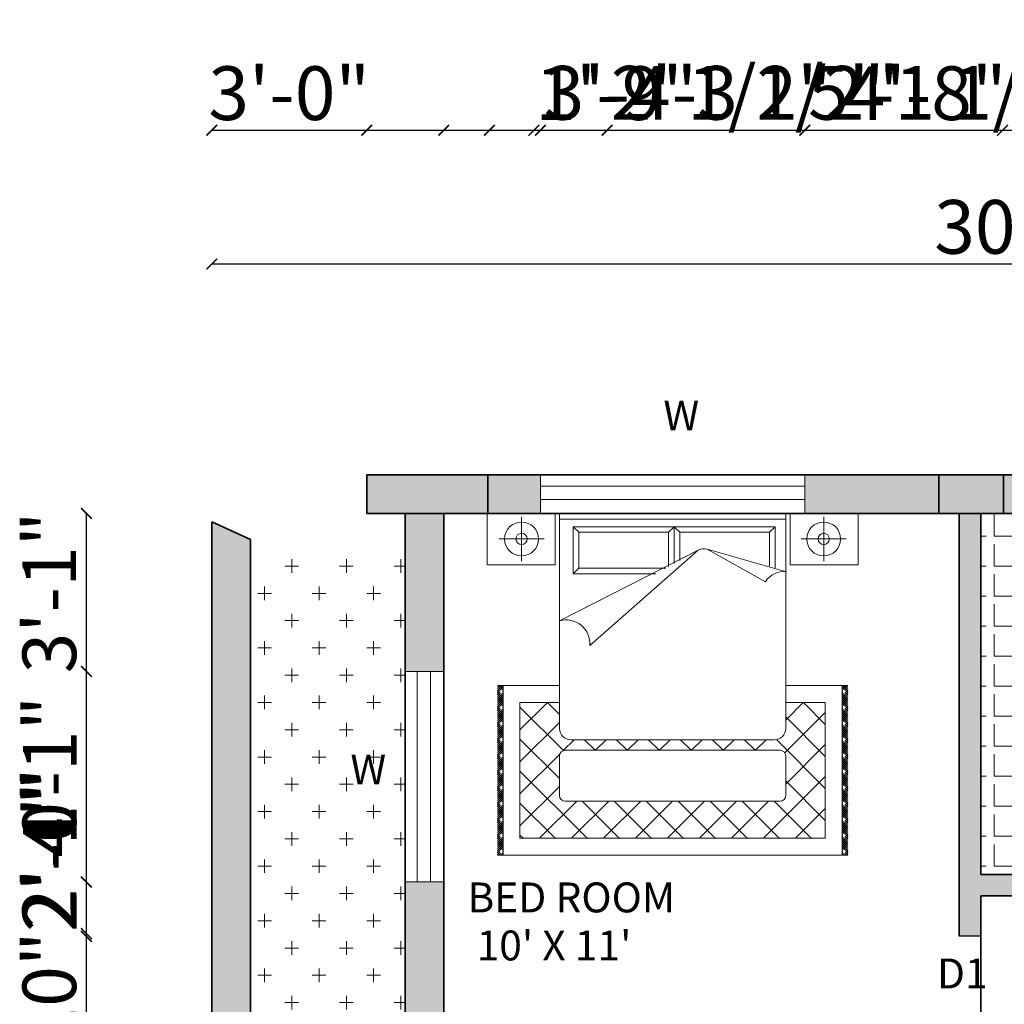
# Model space of a CAD drawing. Units: inches. Extents: x 1858 to 2399, y 1317 to 1943.
# Tile 3 of 8: x 1869 to 2098, y 1714 to 1943. Entities that reach past the tile are written whole.
import ezdxf

# ---------------------------------------------------------------- set-up
doc = ezdxf.new("R2010")
doc.units = ezdxf.units.IN
for name, color, linetype, lineweight in [('A-ANNO-DIMS', 2, 'Continuous', 18), ('A-ANNO-TEXT', 7, 'Continuous', 18), ('A-AREA-IDEN', 7, 'Continuous', 18), ('A-COLS', 7, 'Continuous', 35), ('A-COLS-PATT', 5, 'Continuous', 13), ('A-DOOR', 4, 'Continuous', 25), ('A-FLOR-PATT', 8, 'Continuous', 13), ('A-WALL', 7, 'Continuous', 35), ('A-WALL-PATT', 1, 'Continuous', 13), ('beds', 15, 'Continuous', 18), ('L-SITE-PATT', 8, 'Continuous', 13), ('window', 4, 'Continuous', 18)]:
    doc.layers.add(name, color=color, linetype=linetype, lineweight=lineweight)
doc.styles.get("Standard").update_dxf_attribs({"font": 'arial.ttf'})
doc.dimstyles.new('ISO-25', dxfattribs={"dimtxt": 12.5, "dimasz": 2.5, "dimexe": 1.25, "dimexo": 0.625, "dimtad": 1, "dimdec": 0, "dimlunit": 4, "dimtxsty": 'Standard', "dimblk": 'ARCHTICK', "dimcen": 2.5, "dimse1": 1, "dimse2": 1, "dimclrd": 3, "dimclrt": 4, "dimadec": 0, "dimazin": 0, "dimtfac": 1, "dimtdec": 0, "dimtmove": 0, "dimatfit": 3, "dimfxl": 1, "dimarcsym": 0})

# ---------------------------------------------------------------- blocks, each defined once
blk = doc.blocks.new('A$C4CB008C5')
for p, q in [((0, 3.0188), (0.6, 3.0188)), ((0, 2.5688), (0, 3.0188)), ((0.3042, 2.5999), (0.3042, 2.9921)), ((0.6, 3.0188), (0.6, 2.5688)), ((0.6397, 1.1213), (0.6397, 3.0213)), ((0.6397, 3.0213), (2.6397, 3.0213)), ((0.6397, 2.9713), (2.6397, 2.9713)), ((2.6397, 3.0213), (2.6397, 1.1213)), ((3.2794, 3.0188), (2.6794, 3.0188)), ((2.6794, 3.0188), (2.6794, 2.5688)), ((2.9753, 2.5999), (2.9753, 2.9921)), ((3.2794, 2.5688), (3.2794, 3.0188)), ((0.7588, 2.9048), (2.5468, 2.9048)), ((0.7588, 2.4886), (0.7588, 2.9048)), ((0.7588, 2.9048), (0.8088, 2.8548)), ((1.6028, 2.8548), (1.6528, 2.9048)), ((1.6528, 2.9048), (1.6528, 2.5791)), ((1.6528, 2.9048), (1.7028, 2.8548)), ((2.4968, 2.8548), (2.5468, 2.9048)), ((2.5468, 2.9048), (2.5468, 2.5398)), ((0.1057, 2.796), (0.5033, 2.796)), ((0.8088, 2.8548), (1.6028, 2.8548)), ((0.8088, 2.5386), (0.8088, 2.8548)), ((1.6028, 2.8548), (1.6028, 2.5513)), ((1.7028, 2.8548), (1.7028, 2.6069)), ((1.7028, 2.8548), (2.4968, 2.8548)), ((2.4968, 2.8548), (2.4968, 2.5563)), ((3.1738, 2.796), (2.7761, 2.796)), ((1.946, 2.7052), (2.6461, 2.507)), ((1.946, 2.7052), (2.4598, 2.4178)), ((0.6397, 2.0713), (1.866, 2.6977)), ((0.9063, 1.8539), (1.866, 2.6977)), ((0.6, 2.5688), (0, 2.5688)), ((0.8088, 2.5386), (0.7588, 2.4886)), ((1.58, 2.5386), (0.8088, 2.5386)), ((2.6794, 2.5688), (3.2794, 2.5688)), ((1.4901, 2.4886), (0.7588, 2.4886)), ((0.9071, 1.8666), (0.9192, 1.8666)), ((0.0897, 1.5), (0.6397, 1.5)), ((0.0897, 1.491), (0.0987, 1.5)), ((0.0897, 1.4733), (0.1164, 1.5)), ((0.0897, 1.4557), (0.1341, 1.5)), ((0.1397, 1.4602), (0.1081, 1.4917)), ((0.1397, 1.4778), (0.1175, 1.5)), ((0.1397, 1.4955), (0.1352, 1.5)), ((0.1397, 0), (0.1397, 1.5)), ((2.6397, 1.5), (3.1897, 1.5)), ((3.1397, 1.4955), (3.1442, 1.5)), ((3.1397, 1.4778), (3.1619, 1.5)), ((3.1397, 1.5), (3.1397, 0)), ((3.1397, 1.4602), (3.1713, 1.4917)), ((3.1897, 1.4557), (3.1454, 1.5)), ((3.1897, 1.4733), (3.163, 1.5)), ((3.1897, 1.491), (3.1807, 1.5)), ((0.0904, 1.4741), (0.0897, 1.4748)), ((0.0897, 1.438), (0.1258, 1.4741)), ((0.117, 1.4299), (0.0897, 1.4571)), ((0.1397, 1.3894), (0.0897, 1.4394)), ((0.0897, 1.4203), (0.0993, 1.4299)), ((0.1397, 1.3718), (0.0897, 1.4218)), ((0.1397, 1.3541), (0.0897, 1.4041)), ((0.0897, 1.3496), (0.1397, 1.3996)), ((0.0904, 1.368), (0.1397, 1.4173)), ((0.117, 1.4122), (0.1397, 1.4349)), ((0.1397, 1.4425), (0.1346, 1.4475)), ((3.1397, 1.4425), (3.1448, 1.4475)), ((3.1397, 1.3894), (3.1897, 1.4394)), ((3.1625, 1.4122), (3.1397, 1.4349)), ((3.1397, 1.3718), (3.1897, 1.4218)), ((3.189, 1.368), (3.1397, 1.4173)), ((3.1397, 1.3541), (3.1897, 1.4041)), ((3.1897, 1.3496), (3.1397, 1.3996)), ((3.1897, 1.438), (3.1536, 1.4741)), ((3.1625, 1.4299), (3.1897, 1.4571)), ((3.1897, 1.4203), (3.1801, 1.4299)), ((3.189, 1.4741), (3.1897, 1.4748)), ((0.1397, 1.3364), (0.0897, 1.3864)), ((0.0897, 1.3319), (0.1397, 1.3819)), ((0.0897, 1.3142), (0.1397, 1.3642)), ((0.0904, 1.3326), (0.0897, 1.3334)), ((0.0897, 1.2966), (0.1258, 1.3326)), ((0.117, 1.2885), (0.0897, 1.3157)), ((0.1397, 1.3187), (0.1081, 1.3503)), ((0.1397, 1.3011), (0.1346, 1.3061)), ((0.2897, 1.1076), (0.5321, 1.35)), ((0.2897, 0.15), (0.2897, 1.35)), ((0.2897, 1.35), (0.6397, 1.35)), ((0.6743, 0.9255), (0.2897, 1.3102)), ((0.6397, 1.243), (0.5327, 1.35)), ((2.6397, 1.1949), (2.7948, 1.35)), ((2.6397, 1.35), (2.9897, 1.35)), ((2.9897, 1.1557), (2.7955, 1.35)), ((2.9897, 1.35), (2.9897, 0.15)), ((3.1397, 1.3364), (3.1897, 1.3864)), ((3.1897, 1.3319), (3.1397, 1.3819)), ((3.1897, 1.3142), (3.1397, 1.3642)), ((3.1397, 1.3187), (3.1713, 1.3503)), ((3.1397, 1.3011), (3.1448, 1.3061)), ((3.1897, 1.2966), (3.1536, 1.3326)), ((3.1625, 1.2885), (3.1897, 1.3157)), ((3.189, 1.3326), (3.1897, 1.3334)), ((0.1397, 1.248), (0.0897, 1.298)), ((0.0897, 1.2789), (0.0993, 1.2885)), ((0.1397, 1.2303), (0.0897, 1.2803)), ((0.1397, 1.2127), (0.0897, 1.2627)), ((0.0897, 1.2082), (0.1397, 1.2582)), ((0.1397, 1.195), (0.0897, 1.245)), ((0.0897, 1.1905), (0.1397, 1.2405)), ((0.0897, 1.1728), (0.1397, 1.2228)), ((0.0904, 1.2266), (0.1397, 1.2758)), ((0.117, 1.2708), (0.1397, 1.2935)), ((2.6321, 0.9045), (2.9897, 1.2621)), ((2.9897, 0.8729), (2.6397, 1.2229)), ((3.1397, 1.248), (3.1897, 1.298)), ((3.1625, 1.2708), (3.1397, 1.2935)), ((3.1397, 1.2303), (3.1897, 1.2803)), ((3.189, 1.2266), (3.1397, 1.2758)), ((3.1397, 1.2127), (3.1897, 1.2627)), ((3.1897, 1.2082), (3.1397, 1.2582)), ((3.1397, 1.195), (3.1897, 1.245)), ((3.1897, 1.1905), (3.1397, 1.2405)), ((3.1897, 1.1728), (3.1397, 1.2228)), ((3.1897, 1.2789), (3.1801, 1.2885)), ((0.0904, 1.1912), (0.0897, 1.192)), ((0.0897, 1.1551), (0.1258, 1.1912)), ((0.117, 1.147), (0.0897, 1.1743)), ((0.1397, 1.1066), (0.0897, 1.1566)), ((0.0897, 1.1375), (0.0993, 1.147)), ((0.1397, 1.0889), (0.0897, 1.1389)), ((0.0904, 1.0852), (0.1397, 1.1344)), ((0.1397, 1.1773), (0.1081, 1.2089)), ((0.117, 1.1294), (0.1397, 1.1521)), ((0.1397, 1.1596), (0.1346, 1.1647)), ((0.2897, 0.8248), (0.6397, 1.1748)), ((3.1397, 1.1773), (3.1713, 1.2089)), ((3.1397, 1.1596), (3.1448, 1.1647)), ((3.1397, 1.1066), (3.1897, 1.1566)), ((3.1625, 1.1294), (3.1397, 1.1521)), ((3.1397, 1.0889), (3.1897, 1.1389)), ((3.189, 1.0852), (3.1397, 1.1344)), ((3.1897, 1.1551), (3.1536, 1.1912)), ((3.1625, 1.147), (3.1897, 1.1743)), ((3.1897, 1.1375), (3.1801, 1.147)), ((3.189, 1.1912), (3.1897, 1.192)), ((0.1397, 1.0712), (0.0897, 1.1212)), ((0.0897, 1.0667), (0.1397, 1.1167)), ((0.1397, 1.0536), (0.0897, 1.1036)), ((0.0897, 1.0491), (0.1397, 1.0991)), ((0.0897, 1.0314), (0.1397, 1.0814)), ((0.0904, 1.0498), (0.0897, 1.0505)), ((0.0897, 1.0137), (0.1258, 1.0498)), ((0.1397, 1.0359), (0.1081, 1.0675)), ((3.1397, 1.0712), (3.1897, 1.1212)), ((3.1897, 1.0667), (3.1397, 1.1167)), ((3.1397, 1.0536), (3.1897, 1.1036)), ((3.1897, 1.0491), (3.1397, 1.0991)), ((3.1897, 1.0314), (3.1397, 1.0814)), ((3.1397, 1.0359), (3.1713, 1.0675)), ((3.1897, 1.0137), (3.1536, 1.0498)), ((3.189, 1.0498), (3.1897, 1.0505)), ((0.117, 1.0056), (0.0897, 1.0329)), ((0.1397, 0.9652), (0.0897, 1.0152)), ((0.0897, 0.996), (0.0993, 1.0056)), ((0.1397, 0.9475), (0.0897, 0.9975)), ((0.1397, 0.9298), (0.0897, 0.9798)), ((0.0897, 0.9253), (0.1397, 0.9753)), ((0.1397, 0.9121), (0.0897, 0.9621)), ((0.0904, 0.9437), (0.1397, 0.993)), ((0.117, 0.9879), (0.1397, 1.0107)), ((0.1397, 1.0182), (0.1346, 1.0233)), ((0.6397, 0.6773), (0.2897, 1.0273)), ((0.6727, 0.925), (0.769, 1.0213)), ((2.5397, 1.0213), (0.7397, 1.0213)), ((0.9548, 0.9279), (0.8614, 1.0213)), ((0.9585, 0.9279), (1.0519, 1.0213)), ((1.2376, 0.9279), (1.1443, 1.0213)), ((1.2414, 0.9279), (1.3347, 1.0213)), ((1.5205, 0.9279), (1.4271, 1.0213)), ((1.5242, 0.9279), (1.6176, 1.0213)), ((1.8033, 0.9279), (1.71, 1.0213)), ((1.8071, 0.9279), (1.9004, 1.0213)), ((2.0861, 0.9279), (1.9928, 1.0213)), ((2.0899, 0.9279), (2.1832, 1.0213)), ((2.369, 0.9279), (2.2757, 1.0213)), ((2.3727, 0.9279), (2.4661, 1.0213)), ((2.9897, 0.5901), (2.557, 1.0228)), ((2.6397, 0.6292), (2.9897, 0.9792)), ((3.1397, 1.0182), (3.1448, 1.0233)), ((3.1397, 0.9652), (3.1897, 1.0152)), ((3.1625, 0.9879), (3.1397, 1.0107)), ((3.1397, 0.9475), (3.1897, 0.9975)), ((3.189, 0.9437), (3.1397, 0.993)), ((3.1397, 0.9298), (3.1897, 0.9798)), ((3.1897, 0.9253), (3.1397, 0.9753)), ((3.1397, 0.9121), (3.1897, 0.9621)), ((3.1625, 1.0056), (3.1897, 1.0329)), ((3.1897, 0.996), (3.1801, 1.0056)), ((0.0897, 0.9076), (0.1397, 0.9576)), ((0.0897, 0.89), (0.1397, 0.94)), ((0.0904, 0.9084), (0.0897, 0.9091)), ((0.0897, 0.8723), (0.1258, 0.9084)), ((0.117, 0.8642), (0.0897, 0.8914)), ((0.1397, 0.8238), (0.0897, 0.8738)), ((0.1397, 0.8945), (0.1081, 0.9261)), ((0.1397, 0.8768), (0.1346, 0.8819)), ((0.2897, 0.542), (0.6427, 0.8949)), ((0.6397, 0.8779), (0.6397, 0.5279)), ((0.6897, 0.9279), (2.5897, 0.9279)), ((2.6397, 0.8779), (2.6397, 0.5279)), ((3.1897, 0.9076), (3.1397, 0.9576)), ((3.1897, 0.89), (3.1397, 0.94)), ((3.1397, 0.8945), (3.1713, 0.9261)), ((3.1397, 0.8768), (3.1448, 0.8819)), ((3.1397, 0.8238), (3.1897, 0.8738)), ((3.1897, 0.8723), (3.1536, 0.9084)), ((3.1625, 0.8642), (3.1897, 0.8914)), ((3.189, 0.9084), (3.1897, 0.9091)), ((0.0897, 0.8546), (0.0993, 0.8642)), ((0.1397, 0.8061), (0.0897, 0.8561)), ((0.1397, 0.7884), (0.0897, 0.8384)), ((0.0897, 0.7839), (0.1397, 0.8339)), ((0.1397, 0.7707), (0.0897, 0.8207)), ((0.0897, 0.7662), (0.1397, 0.8162)), ((0.0897, 0.7485), (0.1397, 0.7985)), ((0.0904, 0.8023), (0.1397, 0.8516)), ((0.1397, 0.7531), (0.1081, 0.7846)), ((0.117, 0.8465), (0.1397, 0.8693)), ((3.1625, 0.8465), (3.1397, 0.8693)), ((3.1397, 0.8061), (3.1897, 0.8561)), ((3.189, 0.8023), (3.1397, 0.8516)), ((3.1397, 0.7884), (3.1897, 0.8384)), ((3.1897, 0.7839), (3.1397, 0.8339)), ((3.1397, 0.7707), (3.1897, 0.8207)), ((3.1897, 0.7662), (3.1397, 0.8162)), ((3.1897, 0.7485), (3.1397, 0.7985)), ((3.1397, 0.7531), (3.1713, 0.7846)), ((3.1897, 0.8546), (3.1801, 0.8642)), ((0.0904, 0.767), (0.0897, 0.7677)), ((0.0897, 0.7309), (0.1258, 0.767)), ((0.117, 0.7228), (0.0897, 0.75)), ((0.1397, 0.6823), (0.0897, 0.7323)), ((0.0897, 0.7132), (0.0993, 0.7228)), ((0.1397, 0.6647), (0.0897, 0.7147)), ((0.1397, 0.647), (0.0897, 0.697)), ((0.0904, 0.6609), (0.1397, 0.7102)), ((0.117, 0.7051), (0.1397, 0.7278)), ((0.1397, 0.7354), (0.1346, 0.7404)), ((0.8842, 0.15), (0.2897, 0.7445)), ((3.1397, 0.7354), (3.1448, 0.7404)), ((3.1397, 0.6823), (3.1897, 0.7323)), ((3.1625, 0.7051), (3.1397, 0.7278)), ((3.1397, 0.6647), (3.1897, 0.7147)), ((3.189, 0.6609), (3.1397, 0.7102)), ((3.1397, 0.647), (3.1897, 0.697)), ((3.1897, 0.7309), (3.1536, 0.767)), ((3.1625, 0.7228), (3.1897, 0.75)), ((3.1897, 0.7132), (3.1801, 0.7228)), ((3.189, 0.767), (3.1897, 0.7677)), ((0.0897, 0.6425), (0.1397, 0.6925)), ((0.1397, 0.6293), (0.0897, 0.6793)), ((0.0897, 0.6248), (0.1397, 0.6748)), ((0.0897, 0.6071), (0.1397, 0.6571)), ((0.0904, 0.6255), (0.0897, 0.6263)), ((0.0897, 0.5894), (0.1258, 0.6255)), ((0.1397, 0.6116), (0.1081, 0.6432)), ((2.4433, 0.15), (2.9897, 0.6964)), ((2.9897, 0.3072), (2.6397, 0.6572)), ((3.1897, 0.6425), (3.1397, 0.6925)), ((3.1397, 0.6293), (3.1897, 0.6793)), ((3.1897, 0.6248), (3.1397, 0.6748)), ((3.1897, 0.6071), (3.1397, 0.6571)), ((3.1397, 0.6116), (3.1713, 0.6432)), ((3.1897, 0.5894), (3.1536, 0.6255)), ((3.189, 0.6255), (3.1897, 0.6263)), ((0.117, 0.5813), (0.0897, 0.6086)), ((0.1397, 0.5409), (0.0897, 0.5909)), ((0.0897, 0.5718), (0.0993, 0.5813)), ((0.1397, 0.5232), (0.0897, 0.5732)), ((0.1397, 0.5056), (0.0897, 0.5556)), ((0.0897, 0.5011), (0.1397, 0.5511)), ((0.1397, 0.4879), (0.0897, 0.5379)), ((0.0897, 0.4834), (0.1397, 0.5334)), ((0.0904, 0.5195), (0.1397, 0.5687)), ((0.117, 0.5637), (0.1397, 0.5864)), ((0.1397, 0.594), (0.1346, 0.599)), ((0.2897, 0.2591), (0.6397, 0.6091)), ((3.1397, 0.594), (3.1448, 0.599)), ((3.1397, 0.5409), (3.1897, 0.5909)), ((3.1625, 0.5637), (3.1397, 0.5864)), ((3.1397, 0.5232), (3.1897, 0.5732)), ((3.189, 0.5195), (3.1397, 0.5687)), ((3.1397, 0.5056), (3.1897, 0.5556)), ((3.1897, 0.5011), (3.1397, 0.5511)), ((3.1397, 0.4879), (3.1897, 0.5379)), ((3.1897, 0.4834), (3.1397, 0.5334)), ((3.1625, 0.5813), (3.1897, 0.6086)), ((3.1897, 0.5718), (3.1801, 0.5813)), ((0.0897, 0.4657), (0.1397, 0.5157)), ((0.0904, 0.4841), (0.0897, 0.4849)), ((0.0897, 0.448), (0.1258, 0.4841)), ((0.117, 0.4399), (0.0897, 0.4672)), ((0.1397, 0.3995), (0.0897, 0.4495)), ((0.0897, 0.4303), (0.0993, 0.4399)), ((0.1397, 0.4702), (0.1081, 0.5018)), ((0.117, 0.4222), (0.1397, 0.445)), ((0.1397, 0.4525), (0.1346, 0.4576)), ((0.6013, 0.15), (0.2897, 0.4616)), ((0.4634, 0.15), (0.7914, 0.4779)), ((0.6897, 0.4779), (2.5897, 0.4779)), ((0.7463, 0.15), (1.0742, 0.4779)), ((1.167, 0.15), (0.8391, 0.4779)), ((1.0291, 0.15), (1.3571, 0.4779)), ((1.4499, 0.15), (1.1219, 0.4779)), ((1.312, 0.15), (1.6399, 0.4779)), ((1.7327, 0.15), (1.4048, 0.4779)), ((1.5948, 0.15), (1.9227, 0.4779)), ((2.0156, 0.15), (1.6876, 0.4779)), ((1.8777, 0.15), (2.2056, 0.4779)), ((2.2984, 0.15), (1.9705, 0.4779)), ((2.1605, 0.15), (2.4884, 0.4779)), ((2.5812, 0.15), (2.2533, 0.4779)), ((2.8641, 0.15), (2.5361, 0.4779)), ((3.1897, 0.4657), (3.1397, 0.5157)), ((3.1397, 0.4702), (3.1713, 0.5018)), ((3.1397, 0.4525), (3.1448, 0.4576)), ((3.1397, 0.3995), (3.1897, 0.4495)), ((3.1625, 0.4222), (3.1397, 0.445)), ((3.1897, 0.448), (3.1536, 0.4841)), ((3.1625, 0.4399), (3.1897, 0.4672)), ((3.1897, 0.4303), (3.1801, 0.4399)), ((3.189, 0.4841), (3.1897, 0.4849)), ((0.1397, 0.3818), (0.0897, 0.4318)), ((0.1397, 0.3641), (0.0897, 0.4141)), ((0.0897, 0.3596), (0.1397, 0.4096)), ((0.1397, 0.3465), (0.0897, 0.3965)), ((0.0897, 0.342), (0.1397, 0.392)), ((0.0897, 0.3243), (0.1397, 0.3743)), ((0.0904, 0.3781), (0.1397, 0.4273)), ((0.1397, 0.3288), (0.1081, 0.3604)), ((2.7262, 0.15), (2.9897, 0.4135)), ((3.1397, 0.3818), (3.1897, 0.4318)), ((3.189, 0.3781), (3.1397, 0.4273)), ((3.1397, 0.3641), (3.1897, 0.4141)), ((3.1897, 0.3596), (3.1397, 0.4096)), ((3.1397, 0.3465), (3.1897, 0.3965)), ((3.1897, 0.342), (3.1397, 0.392)), ((3.1897, 0.3243), (3.1397, 0.3743)), ((3.1397, 0.3288), (3.1713, 0.3604)), ((0.0904, 0.3427), (0.0897, 0.3434)), ((0.0897, 0.3066), (0.1258, 0.3427)), ((0.117, 0.2985), (0.0897, 0.3258)), ((0.1397, 0.2581), (0.0897, 0.3081)), ((0.0897, 0.2889), (0.0993, 0.2985)), ((0.1397, 0.2404), (0.0897, 0.2904)), ((0.1397, 0.2227), (0.0897, 0.2727)), ((0.0897, 0.2182), (0.1397, 0.2682)), ((0.0904, 0.2366), (0.1397, 0.2859)), ((0.117, 0.2808), (0.1397, 0.3036)), ((0.1397, 0.3111), (0.1346, 0.3162)), ((3.1397, 0.3111), (3.1448, 0.3162)), ((3.1397, 0.2581), (3.1897, 0.3081)), ((3.1625, 0.2808), (3.1397, 0.3036)), ((3.1397, 0.2404), (3.1897, 0.2904)), ((3.189, 0.2366), (3.1397, 0.2859)), ((3.1397, 0.2227), (3.1897, 0.2727)), ((3.1897, 0.2182), (3.1397, 0.2682)), ((3.1897, 0.3066), (3.1536, 0.3427)), ((3.1625, 0.2985), (3.1897, 0.3258)), ((3.1897, 0.2889), (3.1801, 0.2985)), ((3.189, 0.3427), (3.1897, 0.3434)), ((0.1397, 0.205), (0.0897, 0.255)), ((0.0897, 0.2005), (0.1397, 0.2505)), ((0.0897, 0.1829), (0.1397, 0.2329)), ((0.0904, 0.2013), (0.0897, 0.202)), ((0.0897, 0.1652), (0.1258, 0.2013)), ((0.117, 0.1571), (0.0897, 0.1843)), ((0.1397, 0.1874), (0.1081, 0.219)), ((0.1397, 0.1697), (0.1346, 0.1748)), ((0.3185, 0.15), (0.2897, 0.1788)), ((3.1397, 0.205), (3.1897, 0.255)), ((3.1897, 0.2005), (3.1397, 0.2505)), ((3.1897, 0.1829), (3.1397, 0.2329)), ((3.1397, 0.1874), (3.1713, 0.219)), ((3.1397, 0.1697), (3.1448, 0.1748)), ((3.1897, 0.1652), (3.1536, 0.2013)), ((3.1625, 0.1571), (3.1897, 0.1843)), ((3.189, 0.2013), (3.1897, 0.202)), ((0.1397, 0.1167), (0.0897, 0.1667)), ((0.0897, 0.1475), (0.0993, 0.1571)), ((0.1397, 0.099), (0.0897, 0.149)), ((0.1397, 0.0813), (0.0897, 0.1313)), ((0.0897, 0.0768), (0.1397, 0.1268)), ((0.1397, 0.0636), (0.0897, 0.1136)), ((0.0897, 0.0591), (0.1397, 0.1091)), ((0.0897, 0.0414), (0.1397, 0.0914)), ((0.0904, 0.0952), (0.1397, 0.1445)), ((0.117, 0.1394), (0.1397, 0.1621)), ((2.9897, 0.15), (0.2897, 0.15)), ((3.1397, 0.1167), (3.1897, 0.1667)), ((3.1625, 0.1394), (3.1397, 0.1621)), ((3.1397, 0.099), (3.1897, 0.149)), ((3.189, 0.0952), (3.1397, 0.1445)), ((3.1397, 0.0813), (3.1897, 0.1313)), ((3.1897, 0.0768), (3.1397, 0.1268)), ((3.1397, 0.0636), (3.1897, 0.1136)), ((3.1897, 0.0591), (3.1397, 0.1091)), ((3.1897, 0.0414), (3.1397, 0.0914)), ((3.1897, 0.1475), (3.1801, 0.1571)), ((0.0904, 0.0599), (0.0897, 0.0606)), ((0.0897, 0.0238), (0.1258, 0.0599)), ((0.117, 0.0157), (0.0897, 0.0429)), ((0.1149, 0), (0.0897, 0.0252)), ((0.0897, 0.0061), (0.0993, 0.0157)), ((0.0973, 0), (0.0897, 0.0076)), ((0.1397, 0.0459), (0.1081, 0.0775)), ((0.119, 0), (0.1397, 0.0207)), ((0.1397, 0.0283), (0.1346, 0.0333)), ((0.1367, 0), (0.1397, 0.0031)), ((3.1397, 0.0459), (3.1713, 0.0775)), ((3.1397, 0.0283), (3.1448, 0.0333)), ((3.1604, 0), (3.1397, 0.0207)), ((3.1428, 0), (3.1397, 0.0031)), ((3.1897, 0.0238), (3.1536, 0.0599)), ((3.1625, 0.0157), (3.1897, 0.0429)), ((3.1645, 0), (3.1897, 0.0252)), ((3.1897, 0.0061), (3.1801, 0.0157)), ((3.1822, 0), (3.1897, 0.0076)), ((3.189, 0.0599), (3.1897, 0.0606)), ((0.0897, 0), (3.1897, 0))]:
    blk.add_line(p, q)
for centre, radius in [((0.3042, 2.796), 0.15), ((2.9753, 2.796), 0.15), ((0.3042, 2.796), 0.05), ((2.9753, 2.796), 0.05)]:
    blk.add_circle(centre, radius)
for centre, radius, start, end in [((1.9146, 2.6103), 0.1, 71.72145, 119.07986), ((2.626, 2.3098), 0.1982, 84.17255, 146.98891), ((0.7002, 1.8733), 0.207, 354.64216, 106.97752), ((0.7397, 1.1213), 0.1, 180, 270), ((2.5397, 1.1213), 0.1, 270, 0), ((0.6897, 0.8779), 0.05, 90, 180), ((2.5897, 0.8779), 0.05, 0, 90), ((0.6897, 0.5279), 0.05, 180, 270), ((2.5897, 0.5279), 0.05, 270, 0)]:
    blk.add_arc(centre, radius, start, end)
blk = doc.blocks.new('_ArchTick')
at = {"color": 0, "linetype": 'ByBlock', "const_width": 0.15}
blk.add_lwpolyline([(-0.5, -0.5), (0.5, 0.5)], dxfattribs=at)
blk = doc.blocks.new('*D14')
at = {"layer": 'A-ANNO-DIMS', "color": 0, "lineweight": -2, "transparency": 16777216}
blk.add_line((1913.38, 1886.42), (2273.38, 1886.42), dxfattribs=at)
at = {"layer": 'Defpoints', "color": 0, "transparency": 16777216}
for p in [(2273.38, 1886.42), (2273.38, 1827.14), (1913.38, 1826.41)]:
    blk.add_point(p, dxfattribs=at)
at = {"layer": 'A-ANNO-DIMS', "color": 0, "lineweight": -2, "transparency": 16777216, "xscale": 2.5, "yscale": 2.5, "zscale": 2.5, "rotation": 180}
blk.add_blockref('_ArchTick', (1913.38, 1886.42), dxfattribs=at)
at = {"layer": 'A-ANNO-DIMS', "color": 0, "lineweight": -2, "transparency": 16777216, "xscale": 2.5, "yscale": 2.5, "zscale": 2.5}
blk.add_blockref('_ArchTick', (2273.38, 1886.42), dxfattribs=at)
at = {"layer": 'A-ANNO-DIMS', "color": 0, "transparency": 16777216, "insert": (2093.38, 1893.43), "char_height": 12.5, "attachment_point": 5}
blk.add_mtext("30'", dxfattribs=at)
blk = doc.blocks.new('*D27')
at = {"layer": 'A-ANNO-DIMS', "color": 3, "lineweight": -2, "transparency": 16777216}
blk.add_line((1913.38, 1917.54), (1949.42, 1917.54), dxfattribs=at)
at = {"layer": 'Defpoints', "color": 0, "transparency": 16777216}
for p in [(1949.42, 1917.54), (1949.42, 1837.34), (1913.38, 1826.41)]:
    blk.add_point(p, dxfattribs=at)
at = {"layer": 'A-ANNO-DIMS', "color": 3, "lineweight": -2, "transparency": 16777216, "xscale": 2.5, "yscale": 2.5, "zscale": 2.5, "rotation": 180}
blk.add_blockref('_ArchTick', (1913.38, 1917.54), dxfattribs=at)
at = {"layer": 'A-ANNO-DIMS', "color": 3, "lineweight": -2, "transparency": 16777216, "xscale": 2.5, "yscale": 2.5, "zscale": 2.5}
blk.add_blockref('_ArchTick', (1949.42, 1917.54), dxfattribs=at)
at = {"layer": 'A-ANNO-DIMS', "color": 4, "transparency": 16777216, "insert": (1931.4, 1924.55), "char_height": 12.5, "attachment_point": 5}
blk.add_mtext('3\'-0"', dxfattribs=at)
blk = doc.blocks.new('*D31')
at = {"layer": 'A-ANNO-DIMS', "color": 3, "lineweight": -2, "transparency": 16777216}
for p, q in [((1967.38, 1917.54), (1988.35, 1917.54)), ((1988.35, 1917.54), (2024.15, 1917.54))]:
    blk.add_line(p, q, dxfattribs=at)
at = {"layer": 'Defpoints', "color": 0, "transparency": 16777216}
for p in [(1988.35, 1917.54), (1967.38, 1554.34), (1988.35, 1554.34)]:
    blk.add_point(p, dxfattribs=at)
at = {"layer": 'A-ANNO-DIMS', "color": 3, "lineweight": -2, "transparency": 16777216, "xscale": 2.5, "yscale": 2.5, "zscale": 2.5, "rotation": 180}
blk.add_blockref('_ArchTick', (1967.38, 1917.54), dxfattribs=at)
at = {"layer": 'A-ANNO-DIMS', "color": 3, "lineweight": -2, "transparency": 16777216, "xscale": 2.5, "yscale": 2.5, "zscale": 2.5}
blk.add_blockref('_ArchTick', (1988.35, 1917.54), dxfattribs=at)
at = {"layer": 'A-ANNO-DIMS', "color": 4, "transparency": 16777216, "insert": (2007.5, 1924.55), "char_height": 12.5, "attachment_point": 5}
blk.add_mtext('1\'-9"', dxfattribs=at)
blk = doc.blocks.new('*D32')
at = {"layer": 'A-ANNO-DIMS', "color": 3, "lineweight": -2, "transparency": 16777216}
for p, q in [((1949.42, 1917.54), (1989.86, 1917.54)), ((1989.86, 1917.54), (2055.96, 1917.54))]:
    blk.add_line(p, q, dxfattribs=at)
at = {"layer": 'Defpoints', "color": 0, "transparency": 16777216}
for p in [(1989.86, 1917.54), (1949.42, 1837.34), (1989.86, 1837.34)]:
    blk.add_point(p, dxfattribs=at)
at = {"layer": 'A-ANNO-DIMS', "color": 3, "lineweight": -2, "transparency": 16777216, "xscale": 2.5, "yscale": 2.5, "zscale": 2.5, "rotation": 180}
blk.add_blockref('_ArchTick', (1949.42, 1917.54), dxfattribs=at)
at = {"layer": 'A-ANNO-DIMS', "color": 3, "lineweight": -2, "transparency": 16777216, "xscale": 2.5, "yscale": 2.5, "zscale": 2.5}
blk.add_blockref('_ArchTick', (1989.86, 1917.54), dxfattribs=at)
at = {"layer": 'A-ANNO-DIMS', "color": 4, "transparency": 16777216, "insert": (2024.16, 1924.63), "char_height": 12.5, "attachment_point": 5}
blk.add_mtext('3\'-4 1/2"', dxfattribs=at)
blk = doc.blocks.new('*D33')
at = {"layer": 'A-ANNO-DIMS', "color": 3, "lineweight": -2, "transparency": 16777216}
for p, q in [((1989.86, 1917.54), (2051.43, 1917.54)), ((2051.43, 1917.54), (2117.53, 1917.54))]:
    blk.add_line(p, q, dxfattribs=at)
at = {"layer": 'Defpoints', "color": 0, "transparency": 16777216}
for p in [(2051.43, 1917.54), (1989.86, 1837.34), (2051.43, 1837.34)]:
    blk.add_point(p, dxfattribs=at)
at = {"layer": 'A-ANNO-DIMS', "color": 3, "lineweight": -2, "transparency": 16777216, "xscale": 2.5, "yscale": 2.5, "zscale": 2.5, "rotation": 180}
blk.add_blockref('_ArchTick', (1989.86, 1917.54), dxfattribs=at)
at = {"layer": 'A-ANNO-DIMS', "color": 3, "lineweight": -2, "transparency": 16777216, "xscale": 2.5, "yscale": 2.5, "zscale": 2.5}
blk.add_blockref('_ArchTick', (2051.43, 1917.54), dxfattribs=at)
at = {"layer": 'A-ANNO-DIMS', "color": 4, "transparency": 16777216, "insert": (2085.73, 1924.63), "char_height": 12.5, "attachment_point": 5}
blk.add_mtext('5\'-1 1/2"', dxfattribs=at)
blk = doc.blocks.new('*D34')
at = {"layer": 'A-ANNO-DIMS', "color": 3, "lineweight": -2, "transparency": 16777216}
blk.add_line((2051.43, 1917.54), (2107.67, 1917.54), dxfattribs=at)
at = {"layer": 'Defpoints', "color": 0, "transparency": 16777216}
for p in [(2107.67, 1917.54), (2051.43, 1837.34), (2107.67, 1837.34)]:
    blk.add_point(p, dxfattribs=at)
at = {"layer": 'A-ANNO-DIMS', "color": 3, "lineweight": -2, "transparency": 16777216, "xscale": 2.5, "yscale": 2.5, "zscale": 2.5, "rotation": 180}
blk.add_blockref('_ArchTick', (2051.43, 1917.54), dxfattribs=at)
at = {"layer": 'A-ANNO-DIMS', "color": 3, "lineweight": -2, "transparency": 16777216, "xscale": 2.5, "yscale": 2.5, "zscale": 2.5}
blk.add_blockref('_ArchTick', (2107.67, 1917.54), dxfattribs=at)
at = {"layer": 'A-ANNO-DIMS', "color": 4, "transparency": 16777216, "insert": (2079.55, 1924.55), "char_height": 12.5, "attachment_point": 5}
blk.add_mtext('4\'-8"', dxfattribs=at)
blk = doc.blocks.new('*D45')
at = {"layer": 'A-ANNO-DIMS', "color": 3, "lineweight": -2, "transparency": 16777216}
blk.add_line((1884.18, 1672.42), (1884.18, 1742.58), dxfattribs=at)
at = {"layer": 'Defpoints', "color": 0, "transparency": 16777216}
for p in [(1884.18, 1742.58), (1958.38, 1742.58), (1958.38, 1672.42)]:
    blk.add_point(p, dxfattribs=at)
at = {"layer": 'A-ANNO-DIMS', "color": 3, "lineweight": -2, "transparency": 16777216, "xscale": 2.5, "yscale": 2.5, "zscale": 2.5}
for p, rotation in [((1884.18, 1742.58), 90), ((1884.18, 1672.42), 270)]:
    blk.add_blockref('_ArchTick', p, dxfattribs=dict(at, rotation=rotation))
at = {"layer": 'A-ANNO-DIMS', "color": 4, "transparency": 16777216, "insert": (1877.17, 1707.5), "char_height": 12.5, "attachment_point": 5, "rotation": 90}
blk.add_mtext('5\'-10"', dxfattribs=at)
blk = doc.blocks.new('*D46')
at = {"layer": 'A-ANNO-DIMS', "color": 3, "lineweight": -2, "transparency": 16777216}
blk.add_line((1884.18, 1742.58), (1884.18, 1791.57), dxfattribs=at)
at = {"layer": 'Defpoints', "color": 0, "transparency": 16777216}
for p in [(1884.18, 1791.57), (1958.38, 1791.57), (1958.38, 1742.58)]:
    blk.add_point(p, dxfattribs=at)
at = {"layer": 'A-ANNO-DIMS', "color": 3, "lineweight": -2, "transparency": 16777216, "xscale": 2.5, "yscale": 2.5, "zscale": 2.5}
for p, rotation in [((1884.18, 1791.57), 90), ((1884.18, 1742.58), 270)]:
    blk.add_blockref('_ArchTick', p, dxfattribs=dict(at, rotation=rotation))
at = {"layer": 'A-ANNO-DIMS', "color": 4, "transparency": 16777216, "insert": (1877.28, 1767.08), "char_height": 12.5, "attachment_point": 5, "rotation": 90}
blk.add_mtext('4\'-1"', dxfattribs=at)
blk = doc.blocks.new('*D47')
at = {"layer": 'A-ANNO-DIMS', "color": 3, "lineweight": -2, "transparency": 16777216}
blk.add_line((1884.18, 1791.57), (1884.18, 1828.34), dxfattribs=at)
at = {"layer": 'Defpoints', "color": 0, "transparency": 16777216}
for p in [(1884.18, 1828.34), (1958.38, 1828.34), (1958.38, 1791.57)]:
    blk.add_point(p, dxfattribs=at)
at = {"layer": 'A-ANNO-DIMS', "color": 3, "lineweight": -2, "transparency": 16777216, "xscale": 2.5, "yscale": 2.5, "zscale": 2.5}
for p, rotation in [((1884.18, 1828.34), 90), ((1884.18, 1791.57), 270)]:
    blk.add_blockref('_ArchTick', p, dxfattribs=dict(at, rotation=rotation))
at = {"layer": 'A-ANNO-DIMS', "color": 4, "transparency": 16777216, "insert": (1877.16, 1809.96), "char_height": 12.5, "attachment_point": 5, "rotation": 90}
blk.add_mtext('3\'-1"', dxfattribs=at)
blk = doc.blocks.new('*D50')
at = {"layer": 'A-ANNO-DIMS', "color": 3, "lineweight": -2, "transparency": 16777216}
for p, q in [((2097.46, 1917.54), (2127.41, 1917.54)), ((2127.41, 1917.54), (2164.6, 1917.54))]:
    blk.add_line(p, q, dxfattribs=at)
at = {"layer": 'Defpoints', "color": 0, "transparency": 16777216}
for p in [(2127.41, 1917.54), (2097.46, 1563.34), (2127.41, 1563.34)]:
    blk.add_point(p, dxfattribs=at)
at = {"layer": 'A-ANNO-DIMS', "color": 3, "lineweight": -2, "transparency": 16777216, "xscale": 2.5, "yscale": 2.5, "zscale": 2.5, "rotation": 180}
blk.add_blockref('_ArchTick', (2097.46, 1917.54), dxfattribs=at)
at = {"layer": 'A-ANNO-DIMS', "color": 3, "lineweight": -2, "transparency": 16777216, "xscale": 2.5, "yscale": 2.5, "zscale": 2.5}
blk.add_blockref('_ArchTick', (2127.41, 1917.54), dxfattribs=at)
at = {"layer": 'A-ANNO-DIMS', "color": 4, "transparency": 16777216, "insert": (2147.25, 1924.55), "char_height": 12.5, "attachment_point": 5}
blk.add_mtext('2\'-6"', dxfattribs=at)
blk = doc.blocks.new('*D56')
at = {"layer": 'A-ANNO-DIMS', "color": 3, "lineweight": -2, "transparency": 16777216}
for p, q in [((1977.99, 1917.54), (2005.38, 1917.54)), ((2005.38, 1917.54), (2071.7, 1917.54))]:
    blk.add_line(p, q, dxfattribs=at)
at = {"layer": 'Defpoints', "color": 0, "transparency": 16777216}
for p in [(2005.38, 1917.54), (1977.99, 1696.34), (2005.38, 1696.34)]:
    blk.add_point(p, dxfattribs=at)
at = {"layer": 'A-ANNO-DIMS', "color": 3, "lineweight": -2, "transparency": 16777216, "xscale": 2.5, "yscale": 2.5, "zscale": 2.5, "rotation": 180}
blk.add_blockref('_ArchTick', (1977.99, 1917.54), dxfattribs=at)
at = {"layer": 'A-ANNO-DIMS', "color": 3, "lineweight": -2, "transparency": 16777216, "xscale": 2.5, "yscale": 2.5, "zscale": 2.5}
blk.add_blockref('_ArchTick', (2005.38, 1917.54), dxfattribs=at)
at = {"layer": 'A-ANNO-DIMS', "color": 4, "transparency": 16777216, "insert": (2039.79, 1924.63), "char_height": 12.5, "attachment_point": 5}
blk.add_mtext('2\'-3 1/2"', dxfattribs=at)
blk = doc.blocks.new('*D57')
at = {"layer": 'A-ANNO-DIMS', "color": 3, "lineweight": -2, "transparency": 16777216}
for p, q in [((1884.18, 1729.93), (1884.18, 1767.12)), ((1884.18, 1705.02), (1884.18, 1729.93))]:
    blk.add_line(p, q, dxfattribs=at)
at = {"layer": 'Defpoints', "color": 0, "transparency": 16777216}
for p in [(1884.18, 1729.93), (2087.38, 1729.93), (2087.38, 1705.02)]:
    blk.add_point(p, dxfattribs=at)
at = {"layer": 'A-ANNO-DIMS', "color": 3, "lineweight": -2, "transparency": 16777216, "xscale": 2.5, "yscale": 2.5, "zscale": 2.5}
for p, rotation in [((1884.18, 1729.93), 90), ((1884.18, 1705.02), 270)]:
    blk.add_blockref('_ArchTick', p, dxfattribs=dict(at, rotation=rotation))
at = {"layer": 'A-ANNO-DIMS', "color": 4, "transparency": 16777216, "insert": (1877.28, 1749.77), "char_height": 12.5, "attachment_point": 5, "rotation": 90}
blk.add_mtext('2\'-1"', dxfattribs=at)
blk = doc.blocks.new('*D58')
at = {"layer": 'A-ANNO-DIMS', "color": 3, "lineweight": -2, "transparency": 16777216}
for p, q in [((1884.18, 1730.57), (1884.18, 1767.76)), ((1884.18, 1706.78), (1884.18, 1730.57))]:
    blk.add_line(p, q, dxfattribs=at)
at = {"layer": 'Defpoints', "color": 0, "transparency": 16777216}
for p in [(1884.18, 1730.57), (2145.38, 1730.57), (2145.38, 1706.78)]:
    blk.add_point(p, dxfattribs=at)
at = {"layer": 'A-ANNO-DIMS', "color": 3, "lineweight": -2, "transparency": 16777216, "xscale": 2.5, "yscale": 2.5, "zscale": 2.5}
for p, rotation in [((1884.18, 1730.57), 90), ((1884.18, 1706.78), 270)]:
    blk.add_blockref('_ArchTick', p, dxfattribs=dict(at, rotation=rotation))
at = {"layer": 'A-ANNO-DIMS', "color": 4, "transparency": 16777216, "insert": (1877.17, 1750.41), "char_height": 12.5, "attachment_point": 5, "rotation": 90}
blk.add_mtext('2\'-0"', dxfattribs=at)

msp = doc.modelspace()

# ---------------------------------------------------------------- hatches: boundary and pattern name
at = {"layer": 'A-COLS-PATT'}
h = msp.add_hatch(color=256, dxfattribs=at)
h.dxf.hatch_style = 1
h.paths.add_polyline_path([(1977.99, 1696.34), (1967.38, 1696.34), (1967.38, 1700.89), (1958.38, 1700.89), (1958.38, 1685.05), (1967.38, 1685.05), (1967.38, 1691.34), (1977.99, 1691.34)])
h.paths.add_polyline_path([(1967.38, 1571.83), (1958.38, 1571.83), (1958.38, 1559.34), (1967.38, 1559.34)])
h.paths.add_polyline_path([(1977.97, 1476.34), (1967.38, 1476.34), (1967.38, 1482.01), (1958.38, 1474.25), (1958.38, 1467.34), (1967.38, 1467.34)])
h.paths.add_polyline_path([(2096.38, 1473.96), (2087.38, 1481.51), (2087.38, 1476.34), (2084.48, 1476.34), (2089.85, 1467.34), (2096.38, 1467.34)])
h.paths.add_polyline_path([(2273.38, 1837.34), (2265.79, 1837.34), (2258.24, 1828.34), (2264.38, 1828.34), (2264.38, 1823.36), (2273.38, 1827.14)])
h.paths.add_polyline_path([(2097.64, 1837.34), (2082.58, 1837.34), (2082.58, 1828.34), (2097.64, 1828.34)])
h.paths.add_polyline_path([(1977.66, 1837.34), (1949.42, 1837.34), (1949.42, 1828.34), (1977.66, 1828.34)])
at = {"layer": 'A-FLOR-PATT'}
h = msp.add_hatch(dxfattribs=at)
h.set_pattern_fill('ANGLE', color=256)
h.set_pattern_definition([(0, (0, 0), (0, 6.985), [5.08, -1.905]), (90, (0, 0), (-6.985, 4e-16), [5.08, -1.905])])
h.paths.add_polyline_path([(2058.38, 1691.34), (2005.38, 1691.34), (2005.38, 1696.34), (1977.99, 1696.34), (1977.99, 1691.34), (1967.38, 1691.34), (1967.38, 1643.34), (2026.65, 1643.34), (2026.65, 1651.34), (2033.15, 1651.34), (2031.15, 1657.34, -0.501323), (2036.1, 1676.2, -0.132891), (2038.19, 1676.2, -0.501317), (2043.15, 1657.34), (2041.15, 1651.34), (2044.15, 1651.34), (2044.15, 1652.84), (2047.15, 1652.84), (2047.15, 1651.34), (2047.65, 1651.34), (2047.65, 1643.34), (2058.38, 1643.34)])
h.paths.add_polyline_path([(2140.38, 1828.34), (2130, 1828.34), (2130, 1820.34), (2123.5, 1820.34), (2125.5, 1814.34, -0.501323), (2120.55, 1795.48, -0.132891), (2118.46, 1795.48, -0.501317), (2113.5, 1814.34), (2115.5, 1820.34), (2112.5, 1820.34), (2112.5, 1818.84), (2109.5, 1818.84), (2109.5, 1820.34), (2109, 1820.34), (2109, 1828.34), (2107.67, 1828.34), (2092.38, 1828.34), (2092.38, 1744.34), (2140.38, 1744.34)])
h.paths.add_polyline_path([(1981.03, 1683.02), (1996.96, 1683.02), (1996.96, 1693.5), (1981.03, 1693.5)], flags=24)
h.paths.add_polyline_path([(1975.79, 1660.59), (2014.55, 1660.59), (2014.55, 1671.04), (1975.79, 1671.04)], flags=24)
h.paths.add_polyline_path([(1975.73, 1671.6), (2013.37, 1671.6), (2013.37, 1682.41), (1975.73, 1682.41)], flags=24)
h.paths.add_polyline_path([(2096.15, 1778.17), (2126.05, 1778.17), (2126.05, 1788.61), (2096.15, 1788.61)], flags=24)
h.paths.add_polyline_path([(2096.09, 1789.17), (2133.73, 1789.17), (2133.73, 1799.98), (2096.09, 1799.98)], flags=24)
at = {"layer": 'A-WALL-PATT'}
h = msp.add_hatch(color=256, dxfattribs=at)
h.dxf.hatch_style = 1
h.paths.add_polyline_path([(1967.38, 1742.58), (1958.38, 1742.58), (1958.38, 1700.89), (1967.38, 1700.89)])
h.paths.add_polyline_path([(1967.38, 1685.05), (1958.38, 1685.05), (1958.38, 1672.42), (1967.38, 1672.42)], flags=17)
h.paths.add_polyline_path([(2092.38, 1643.34), (2087.38, 1643.34), (2063.38, 1643.34), (2063.38, 1691.34), (2087.38, 1691.34), (2092.38, 1691.34), (2092.38, 1696.34), (2087.38, 1696.34), (2005.38, 1696.34), (2005.38, 1691.34), (2058.38, 1691.34), (2058.38, 1643.34), (1967.38, 1643.34), (1967.38, 1652.51), (1958.38, 1652.51), (1958.38, 1625.4), (1967.38, 1625.4), (1967.38, 1638.34), (2087.38, 1638.34), (2087.38, 1617.63), (2092.38, 1617.63)])
h.paths.add_polyline_path([(1967.38, 1591.74), (1958.38, 1591.74), (1958.38, 1571.83), (1967.38, 1571.83)])
h.paths.add_polyline_path([(1967.38, 1554.34), (2002.1, 1554.34), (2002.1, 1559.34), (1967.38, 1559.34), (1958.38, 1559.34), (1958.38, 1536.07), (1967.38, 1536.07)])
h.paths.add_polyline_path([(2087.38, 1559.34), (2042.3, 1559.34), (2042.3, 1554.34), (2087.38, 1554.34)])
h.paths.add_polyline_path([(2092.38, 1583.24), (2087.38, 1583.24), (2087.38, 1563.34), (2092.38, 1563.34)])
h.paths.add_polyline_path([(2096.38, 1554.34), (2087.38, 1554.34), (2087.38, 1481.51), (2096.38, 1473.96)])
h.paths.add_polyline_path([(2084.48, 1476.34), (2050.44, 1476.34), (2050.44, 1467.34), (2089.85, 1467.34)])
h.paths.add_polyline_path([(2002.33, 1476.34), (1977.97, 1476.34), (1967.38, 1467.34), (2002.33, 1467.34)])
h.paths.add_polyline_path([(1967.38, 1488.33), (1958.38, 1488.33), (1958.38, 1474.25), (1967.38, 1482.01)])
h.paths.add_polyline_path([(2121.99, 1554.34), (2119.71, 1554.34), (2119.71, 1532.61), (2096.38, 1532.61), (2096.38, 1529.65), (2121.99, 1529.65)])
h.paths.add_polyline_path([(2171.86, 1563.34), (2127.41, 1563.34), (2127.41, 1554.34), (2171.86, 1554.34)])
h.paths.add_polyline_path([(2264.38, 1563.34), (2220, 1563.34), (2220, 1554.34), (2264.38, 1554.34)])
h.paths.add_polyline_path([(2273.38, 1563.34), (2264.38, 1563.34), (2264.38, 1366.34), (2241.64, 1366.34), (2241.64, 1357.34), (2273.38, 1357.34)])
h.paths.add_polyline_path([(2273.38, 1691.34), (2264.38, 1691.34), (2264.38, 1576.35), (2273.38, 1576.35)])
h.paths.add_polyline_path([(2273.38, 1827.14), (2264.38, 1823.36), (2264.38, 1706.46), (2273.38, 1706.46)])
h.paths.add_polyline_path([(2265.79, 1837.34), (2234.56, 1837.34), (2234.56, 1828.34), (2258.24, 1828.34)])
h.paths.add_polyline_path([(2186.7, 1837.34), (2131.33, 1837.34), (2131.33, 1828.34), (2186.7, 1828.34)])
h.paths.add_polyline_path([(2107.67, 1837.34), (2097.64, 1837.34), (2097.64, 1828.34), (2107.67, 1828.34)])
h.paths.add_polyline_path([(2082.58, 1837.34), (2051.43, 1837.34), (2051.43, 1828.34), (2082.58, 1828.34)])
h.paths.add_polyline_path([(2092.38, 1828.34), (2087.38, 1828.34), (2087.38, 1729.93), (2092.38, 1729.93), (2092.38, 1739.34), (2140.38, 1739.34), (2140.38, 1730.57), (2145.38, 1730.57), (2145.38, 1828.34), (2140.38, 1828.34), (2140.38, 1744.34), (2092.38, 1744.34)])
h.paths.add_polyline_path([(1989.86, 1837.34), (1977.66, 1837.34), (1977.66, 1828.34), (1989.86, 1828.34)])
h.paths.add_polyline_path([(1922.38, 1822.27), (1913.38, 1826.41), (1913.38, 1357.34), (1951.36, 1357.34), (1951.36, 1366.34), (1922.38, 1366.34)])
h.paths.add_polyline_path([(1967.38, 1828.34), (1958.38, 1828.34), (1958.38, 1791.57), (1967.38, 1791.57)])
at = {"layer": 'L-SITE-PATT'}
h = msp.add_hatch(dxfattribs=at)
h.set_pattern_fill('CROSS', color=256)
h.paths.add_polyline_path([(1958.38, 1820.26), (1922.38, 1820.26), (1922.38, 1366.34), (1958.38, 1366.34), (1958.38, 1389.85), (1945.69, 1389.85), (1945.69, 1424.76), (1958.38, 1424.76)])
h.paths.add_polyline_path([(1943.89, 1763.53), (1956.55, 1763.53), (1956.55, 1773.97), (1943.89, 1773.97)], flags=24)
h.paths.add_polyline_path([(1948.35, 1662.61), (1958.32, 1662.61), (1958.32, 1673.05), (1948.35, 1673.05)], flags=24)
h.paths.add_polyline_path([(1938.82, 1510.71), (1951.47, 1510.71), (1951.47, 1521.15), (1938.82, 1521.15)], flags=24)
h.paths.add_polyline_path([(1939.14, 1601.55), (1951.8, 1601.55), (1951.8, 1611.99), (1939.14, 1611.99)], flags=24)

# ---------------------------------------------------------------- linework, layer by layer
at = {"layer": 'A-COLS'}
for p, q in [((1949.42, 1837.34), (1949.42, 1828.34)), ((1977.66, 1837.34), (1977.66, 1828.34)), ((2082.58, 1837.34), (2082.58, 1828.34)), ((2097.64, 1837.34), (2097.64, 1828.34))]:
    msp.add_line(p, q, dxfattribs=at)
at = {"layer": 'A-DOOR'}
msp.add_line((2092.38, 1729.93), (2087.38, 1729.93), dxfattribs=at)
at = {"layer": 'A-WALL'}
for p, q in [((1949.42, 1828.34), (2264.38, 1828.34)), ((1958.38, 1366.34), (1958.38, 1828.34)), ((1967.38, 1696.34), (1967.38, 1828.34)), ((2087.38, 1729.93), (2087.38, 1828.34)), ((2092.38, 1744.34), (2092.38, 1828.34)), ((1922.38, 1822.27), (1913.38, 1826.41)), ((1922.38, 1366.34), (1922.38, 1822.27)), ((2092.38, 1744.34), (2140.38, 1744.34)), ((2092.38, 1739.34), (2140.38, 1739.34)), ((2092.38, 1696.34), (2092.38, 1739.34))]:
    msp.add_line(p, q, dxfattribs=at)
msp.add_lwpolyline([(1949.42, 1837.34), (2273.38, 1837.34), (2273.38, 1357.34), (1913.38, 1357.34), (1913.38, 1826.41)], dxfattribs=at)
at = {"layer": 'window'}
for p, q in [((1989.86, 1837.34), (1989.86, 1828.34)), ((2051.43, 1837.34), (1989.86, 1837.34)), ((2051.43, 1828.34), (2051.43, 1837.34)), ((2051.43, 1834.73), (1989.86, 1834.73)), ((2051.43, 1831.58), (1989.86, 1831.58)), ((1989.86, 1828.34), (2051.43, 1828.34)), ((1967.38, 1791.57), (1958.38, 1791.57)), ((1958.38, 1791.57), (1958.38, 1742.58)), ((1961.18, 1791.57), (1961.18, 1742.58)), ((1964.31, 1791.57), (1964.31, 1742.58)), ((1967.38, 1742.58), (1967.38, 1791.57)), ((1958.38, 1742.58), (1967.38, 1742.58))]:
    msp.add_line(p, q, dxfattribs=at)

# ---------------------------------------------------------------- block references
at = {"layer": 'beds', "xscale": 26.32639920834102, "yscale": 26.32639920834102, "zscale": 26.32639920834102}
msp.add_blockref('A$C4CB008C5', (1977.48, 1748.8), dxfattribs=at)

# ---------------------------------------------------------------- texts
at = {"layer": 'A-ANNO-TEXT'}
for s, p in [('W', (2018.49, 1847.67)), ('W', (1945.63, 1765.27)), ('D1', (2082.18, 1717.8))]:
    msp.add_text(s, height=6.96, dxfattribs=at).set_placement(p)
at = {"layer": 'A-AREA-IDEN'}
for s, p in [('BED ROOM', (1972.88, 1735.5)), (" 10' X 11'", (1972.88, 1724.32))]:
    msp.add_text(s, height=6.96, dxfattribs=at).set_placement(p)

# ---------------------------------------------------------------- dimensions: what is measured, and where the dimension line sits
at = {"layer": 'A-ANNO-DIMS'}
for base, p1, p2, override, picture, middle in [((1989.86, 1917.54), (1949.42, 1837.34), (1989.86, 1837.34), {"dimdec": 1, "dimlfac": 1, "dimrnd": 0, "dimzin": 1, "dimdsep": 46, "dimlunit": 4, "dimfrac": 2}, '*D32', (2024.16, 1924.63)), ((2005.38, 1917.54), (1977.99, 1696.34), (2005.38, 1696.34), {"dimdec": 1, "dimlfac": 1, "dimrnd": 0, "dimzin": 1, "dimdsep": 46, "dimlunit": 4, "dimfrac": 2}, '*D56', (2039.79, 1924.63)), ((2051.43, 1917.54), (1989.86, 1837.34), (2051.43, 1837.34), {"dimdec": 1, "dimlfac": 1, "dimrnd": 0, "dimzin": 1, "dimdsep": 46, "dimlunit": 4, "dimfrac": 2}, '*D33', (2085.73, 1924.63)), ((1949.42, 1917.54), (1913.38, 1826.41), (1949.42, 1837.34), {"dimdec": 1, "dimlfac": 1, "dimrnd": 0, "dimzin": 1, "dimdsep": 46, "dimlunit": 4, "dimfrac": 2}, '*D27', (1931.4, 1924.55)), ((1988.35, 1917.54), (1967.38, 1554.34), (1988.35, 1554.34), {"dimdec": 1, "dimlfac": 1, "dimrnd": 0, "dimzin": 1, "dimdsep": 46, "dimlunit": 4, "dimfrac": 2}, '*D31', (2007.5, 1924.55)), ((2107.67, 1917.54), (2051.43, 1837.34), (2107.67, 1837.34), {"dimdec": 1, "dimlfac": 1, "dimrnd": 0, "dimzin": 1, "dimdsep": 46, "dimlunit": 4, "dimfrac": 2}, '*D34', (2079.55, 1924.55)), ((2127.4089, 1917.5395), (2097.4626, 1563.3395), (2127.4089, 1563.3395), {"dimdec": 1, "dimlfac": 1, "dimrnd": 0, "dimzin": 1, "dimdsep": 46, "dimlunit": 4, "dimfrac": 2}, '*D50', (2147.2545, 1924.5467)), ((2273.38, 1886.42), (1913.38, 1826.41), (2273.38, 1827.14), {"dimclrd": 0, "dimclre": 0, "dimclrt": 0}, '*D14', (2093.38, 1893.43))]:
    dim = msp.add_linear_dim(base=base, p1=p1, p2=p2, dimstyle='ISO-25', override=override, dxfattribs=at)
    dim.commit()
    dim.dimension.update_dxf_attribs({"geometry": picture, "text_midpoint": middle})
for base, p1, p2, picture, middle in [((1884.18, 1828.34), (1958.38, 1791.57), (1958.38, 1828.34), '*D47', (1877.16, 1809.96)), ((1884.18, 1791.57), (1958.38, 1742.58), (1958.38, 1791.57), '*D46', (1877.28, 1767.08)), ((1884.18, 1730.57), (2145.38, 1706.78), (2145.38, 1730.57), '*D58', (1877.17, 1750.41)), ((1884.18, 1729.93), (2087.38, 1705.02), (2087.38, 1729.93), '*D57', (1877.28, 1749.77)), ((1884.18, 1742.58), (1958.38, 1672.42), (1958.38, 1742.58), '*D45', (1877.17, 1707.5))]:
    dim = msp.add_linear_dim(base=base, p1=p1, p2=p2, angle=90, dimstyle='ISO-25', override={"dimdec": 1, "dimlfac": 1, "dimrnd": 0, "dimzin": 1, "dimdsep": 46, "dimlunit": 4, "dimfrac": 2}, dxfattribs=at)
    dim.commit()
    dim.dimension.update_dxf_attribs({"geometry": picture, "text_midpoint": middle})

doc.saveas('drawing.dxf')
